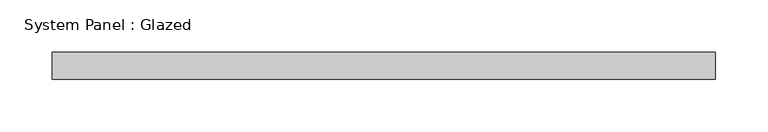
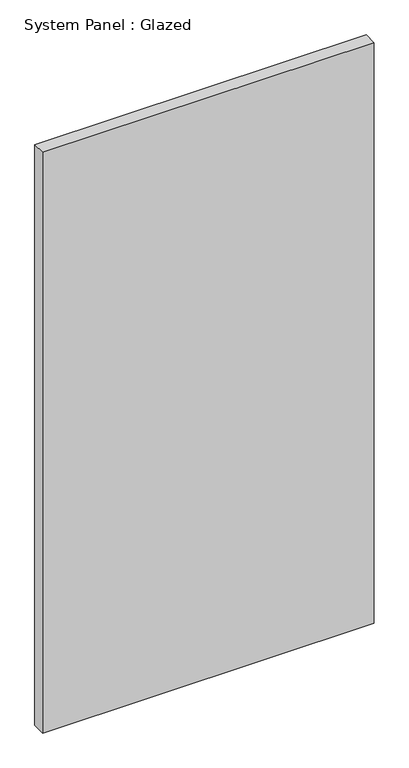
"""IFC4 building model written with IfcOpenShell, lengths in millimetres: plate geometry, System Panel : Glazed."""

from ifc_helpers import new_model, si_unit, origin, origin_with_axes, place, context, project, spatial, polyline, outline, extrude, source, transform, mapped, element, save


def system_panel_glazed_61b33e5d(model_context):
    return source(origin(), model_context, "Body", "SweptSolid", [
        extrude(outline(polyline([(316.4416667, 19.05), (-316.4416667, 19.05), (-316.4416667, 44.45), (316.4416667, 44.45), (316.4416667, 19.05)])), origin_with_axes(), (0.0, 0.0, 1.0), 1171.2581531),
    ])


if __name__ == "__main__":
    model = new_model("IFC4")
    model_context = context("Model", 3, world=origin())
    ifc_project = project(units=[si_unit("LENGTHUNIT", "METRE", prefix="MILLI")], contexts=[model_context])
    site = spatial("IfcSite", under=ifc_project)
    building = spatial("IfcBuilding", under=site)
    placement = place(None, origin())
    system_panel_glazed_shape = system_panel_glazed_61b33e5d(model_context)
    element("IfcPlate", 1, ObjectType="System Panel : Glazed", at=placement, inside=building, context=model_context, shape_type="MappedRepresentation", body=[
        mapped(system_panel_glazed_shape, transform((0.0, 0.0, 0.0), x_axis=(1.0, 0.0, 0.0), y_axis=(0.0, 1.0, 0.0), z_axis=(0.0, 0.0, 1.0))),
    ])
    save(model, "model.ifc")

# Revit data of these elements
# Type "System Panel : Glazed"
#   Construction Type Id = "GSP4R"
#   Analytic Construction = "1/8 in Pilkington single glazing"
#   Visual Light Transmittance = 0.9
#   Solar Heat Gain Coefficient = 0.86
#   Heat Transfer Coefficient (U) = 1.18115 BTU/(h·ft²·°F)
#   Define Thermal Properties by = 1
# Element 1 (IfcPlate, "System Panel : Glazed")
#   Materials on its faces: "Glass"
# Materials
#   "Glass": class "Glass", colour RGB 0 128 192, transparency 0.75, Description = "Soda Lime Glass", Cost = 0
